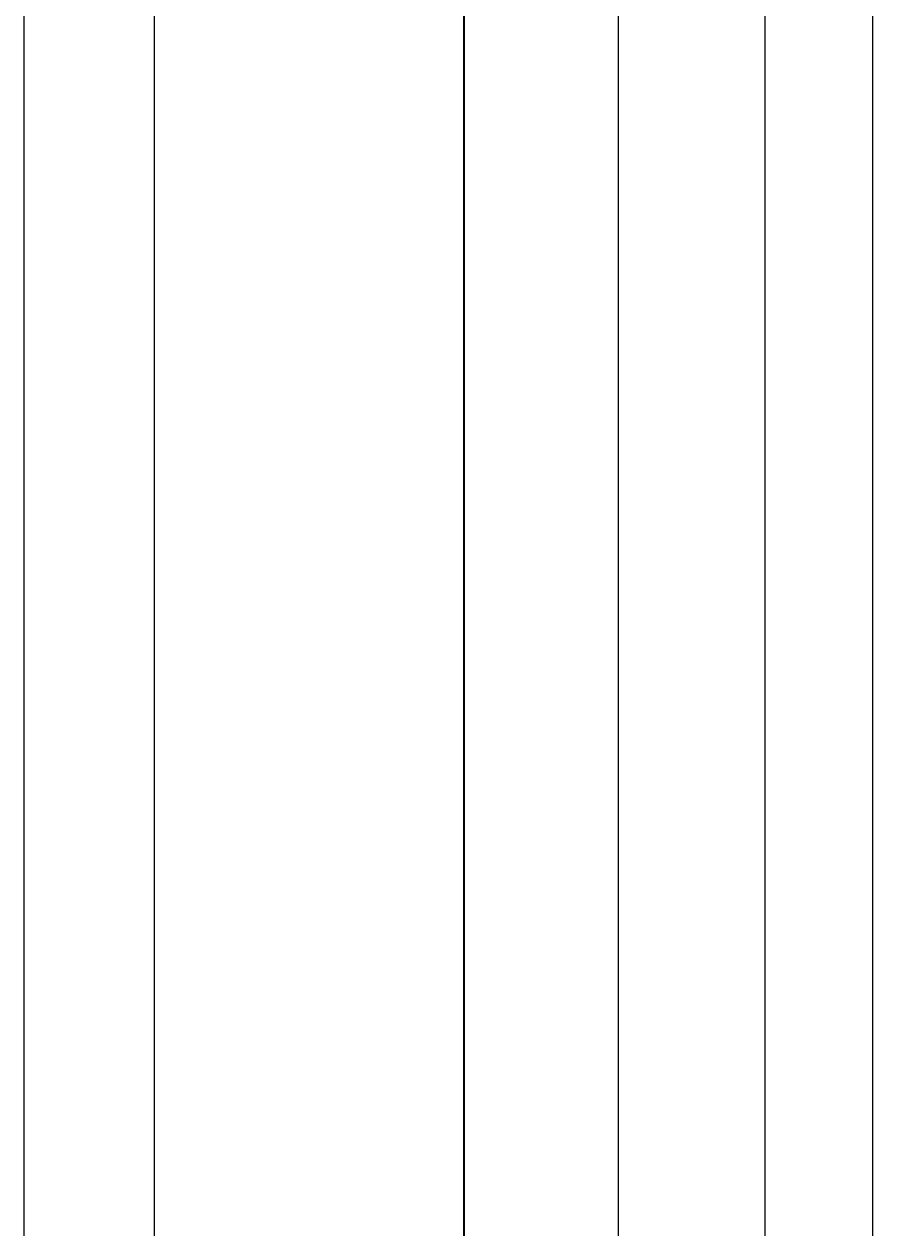
# Model space of a CAD drawing. Units: inches. Extents: x -6 to 289, y -8 to 323.
# Tile 56 of 107: x 107 to 124, y 182 to 206. Entities that reach past the tile are written whole.
import ezdxf

# ---------------------------------------------------------------- set-up
doc = ezdxf.new("R2010")
doc.units = ezdxf.units.IN
doc.header["$MEASUREMENT"] = 0
doc.layers.add('A-ANNO-DIMS', color=2, linetype='Continuous', lineweight=18)
doc.layers.add('A-ELEV', color=7, linetype='Continuous', lineweight=35)
doc.styles.get("Standard").update_dxf_attribs({"font": 'arial.ttf'})
doc.dimstyles.get("Standard").update_dxf_attribs({"dimtxt": 0.18, "dimasz": 0.18, "dimexe": 0.18, "dimexo": 0.0625, "dimgap": 0.09, "dimtad": 0, "dimtih": 1, "dimtoh": 1, "dimdec": 4, "dimzin": 0, "dimdsep": 46, "dimtxsty": 'Standard', "dimcen": 0.09, "dimadec": 0, "dimazin": 0, "dimtfac": 1, "dimtdec": 4, "dimtofl": 0, "dimtmove": 0, "dimatfit": 3, "dimfxl": 1, "dimtolj": 1, "dimtzin": 0, "dimarcsym": 0})

# ---------------------------------------------------------------- blocks, each defined once
blk = doc.blocks.new('*D58')
at = {"layer": 'A-ANNO-DIMS', "color": 0, "lineweight": -2, "transparency": 16777216}
for p, q in [((106.634, 68.495), (106.634, 322.969)), ((106.814, 322.789), (114.479, 322.789)), ((122.914, 322.789), (115.249, 322.789)), ((123.094, 68.495), (123.094, 322.969))]:
    blk.add_line(p, q, dxfattribs=at)
at = {"layer": 'A-ANNO-DIMS', "color": 0, "transparency": 16777216}
for points in [[(106.814, 322.819), (106.814, 322.759), (106.634, 322.789)], [(122.914, 322.819), (122.914, 322.759), (123.094, 322.789)]]:
    blk.add_solid(points, dxfattribs=at)
at = {"layer": 'Defpoints', "color": 0, "transparency": 16777216}
for p in [(123.094, 322.789), (106.634, 68.432), (123.094, 68.432)]:
    blk.add_point(p, dxfattribs=at)
at = {"layer": 'A-ANNO-DIMS', "color": 0, "transparency": 16777216, "insert": (114.864, 322.789), "char_height": 0.18, "attachment_point": 5}
blk.add_mtext('\\A1;16.46', dxfattribs=at)
blk = doc.blocks.new('*D73')
at = {"layer": 'A-ANNO-DIMS', "color": 0, "lineweight": -2, "transparency": 16777216}
for p, q in [((121.008, 51.148), (121.008, 322.969)), ((121.188, 322.789), (127.697, 322.789)), ((135.116, 322.789), (128.607, 322.789)), ((135.296, 51.148), (135.296, 322.969))]:
    blk.add_line(p, q, dxfattribs=at)
at = {"layer": 'A-ANNO-DIMS', "color": 0, "transparency": 16777216}
for points in [[(121.188, 322.819), (121.188, 322.759), (121.008, 322.789)], [(135.116, 322.819), (135.116, 322.759), (135.296, 322.789)]]:
    blk.add_solid(points, dxfattribs=at)
at = {"layer": 'Defpoints', "color": 0, "transparency": 16777216}
for p in [(135.296, 322.789), (121.008, 51.085), (135.296, 51.085)]:
    blk.add_point(p, dxfattribs=at)
at = {"layer": 'A-ANNO-DIMS', "color": 0, "transparency": 16777216, "insert": (128.152, 322.789), "char_height": 0.18, "attachment_point": 5}
blk.add_mtext('\\A1;14.288', dxfattribs=at)
blk = doc.blocks.new('*D92')
at = {"layer": 'A-ANNO-DIMS', "color": 0, "lineweight": -2, "transparency": 16777216}
for p, q in [((109.164, 127.351), (109.164, 322.969)), ((109.344, 322.789), (112.014, 322.789)), ((114.984, 322.789), (112.313, 322.789)), ((115.164, 162.411), (115.164, 322.969))]:
    blk.add_line(p, q, dxfattribs=at)
at = {"layer": 'A-ANNO-DIMS', "color": 0, "transparency": 16777216}
for points in [[(109.344, 322.819), (109.344, 322.759), (109.164, 322.789)], [(114.984, 322.819), (114.984, 322.759), (115.164, 322.789)]]:
    blk.add_solid(points, dxfattribs=at)
at = {"layer": 'Defpoints', "color": 0, "transparency": 16777216}
for p in [(115.164, 322.789), (115.164, 162.348), (109.164, 127.289)]:
    blk.add_point(p, dxfattribs=at)
at = {"layer": 'A-ANNO-DIMS', "color": 0, "transparency": 16777216, "insert": (112.164, 322.789), "char_height": 0.18, "attachment_point": 5}
blk.add_mtext('\\A1;6', dxfattribs=at)
blk = doc.blocks.new('*D93')
at = {"layer": 'A-ANNO-DIMS', "color": 0, "lineweight": -2, "transparency": 16777216}
for p, q in [((115.164, 162.411), (115.164, 322.969)), ((115.344, 322.789), (116.515, 322.789)), ((117.984, 322.789), (116.813, 322.789)), ((118.164, 159.411), (118.164, 322.969))]:
    blk.add_line(p, q, dxfattribs=at)
at = {"layer": 'A-ANNO-DIMS', "color": 0, "transparency": 16777216}
for points in [[(115.344, 322.819), (115.344, 322.759), (115.164, 322.789)], [(117.984, 322.819), (117.984, 322.759), (118.164, 322.789)]]:
    blk.add_solid(points, dxfattribs=at)
at = {"layer": 'Defpoints', "color": 0, "transparency": 16777216}
for p in [(118.164, 322.789), (115.164, 162.348), (118.164, 159.348)]:
    blk.add_point(p, dxfattribs=at)
at = {"layer": 'A-ANNO-DIMS', "color": 0, "transparency": 16777216, "insert": (116.664, 322.789), "char_height": 0.18, "attachment_point": 5}
blk.add_mtext('\\A1;3', dxfattribs=at)
blk = doc.blocks.new('*D94')
at = {"layer": 'A-ANNO-DIMS', "color": 0, "lineweight": -2, "transparency": 16777216}
for p, q in [((118.164, 159.411), (118.164, 322.969)), ((118.344, 322.789), (139.46, 322.789)), ((161.372, 322.789), (140.256, 322.789)), ((161.552, 159.411), (161.552, 322.969))]:
    blk.add_line(p, q, dxfattribs=at)
at = {"layer": 'A-ANNO-DIMS', "color": 0, "transparency": 16777216}
for points in [[(118.344, 322.819), (118.344, 322.759), (118.164, 322.789)], [(161.372, 322.819), (161.372, 322.759), (161.552, 322.789)]]:
    blk.add_solid(points, dxfattribs=at)
at = {"layer": 'Defpoints', "color": 0, "transparency": 16777216}
for p in [(161.552, 322.789), (118.164, 159.348), (161.552, 159.348)]:
    blk.add_point(p, dxfattribs=at)
at = {"layer": 'A-ANNO-DIMS', "color": 0, "transparency": 16777216, "insert": (139.858, 322.789), "char_height": 0.18, "attachment_point": 5}
blk.add_mtext('\\A1;43.39', dxfattribs=at)

msp = doc.modelspace()

# ---------------------------------------------------------------- linework, layer by layer
at = {"layer": 'A-ELEV'}
msp.add_line((115.1638, 247.2888), (115.1638, 139.2888), dxfattribs=at)

# ---------------------------------------------------------------- dimensions: what is measured, and where the dimension line sits
at = {"layer": 'A-ANNO-DIMS'}
for base, p1, p2, override, picture, middle in [((123.094, 322.7888), (106.634, 68.4322), (123.094, 68.4322), {"dimdec": 2, "dimlfac": 1, "dimrnd": 0, "dimzin": 0, "dimdsep": 46, "dimlunit": 2}, '*D58', (114.864, 322.7888)), ((115.1638, 322.7888), (109.1638, 127.2888), (115.1638, 162.3484), {"dimdec": 0, "dimlfac": 1, "dimrnd": 0, "dimzin": 0, "dimdsep": 46, "dimlunit": 2}, '*D92', (112.1638, 322.7888)), ((118.1638, 322.7888), (115.1638, 162.3484), (118.1638, 159.3484), {"dimdec": 0, "dimlfac": 1, "dimrnd": 0, "dimzin": 0, "dimdsep": 46, "dimlunit": 2}, '*D93', (116.6638, 322.7888)), ((161.5522, 322.7888), (118.1638, 159.3484), (161.5522, 159.3484), {"dimdec": 2, "dimlfac": 1, "dimrnd": 0, "dimzin": 0, "dimdsep": 46, "dimlunit": 2}, '*D94', (139.858, 322.7888)), ((135.296, 322.7888), (121.008, 51.0851), (135.296, 51.0851), {"dimdec": 3, "dimlfac": 1, "dimrnd": 0, "dimzin": 0, "dimdsep": 46, "dimlunit": 2}, '*D73', (128.152, 322.7888))]:
    dim = msp.add_linear_dim(base=base, p1=p1, p2=p2, dimstyle='Standard', override=override, dxfattribs=at)
    dim.commit()
    dim.dimension.update_dxf_attribs({"geometry": picture, "text_midpoint": middle})

doc.saveas('drawing.dxf')
